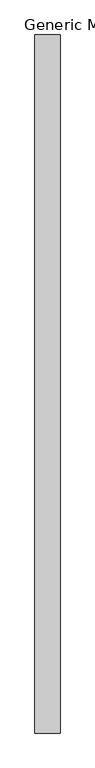
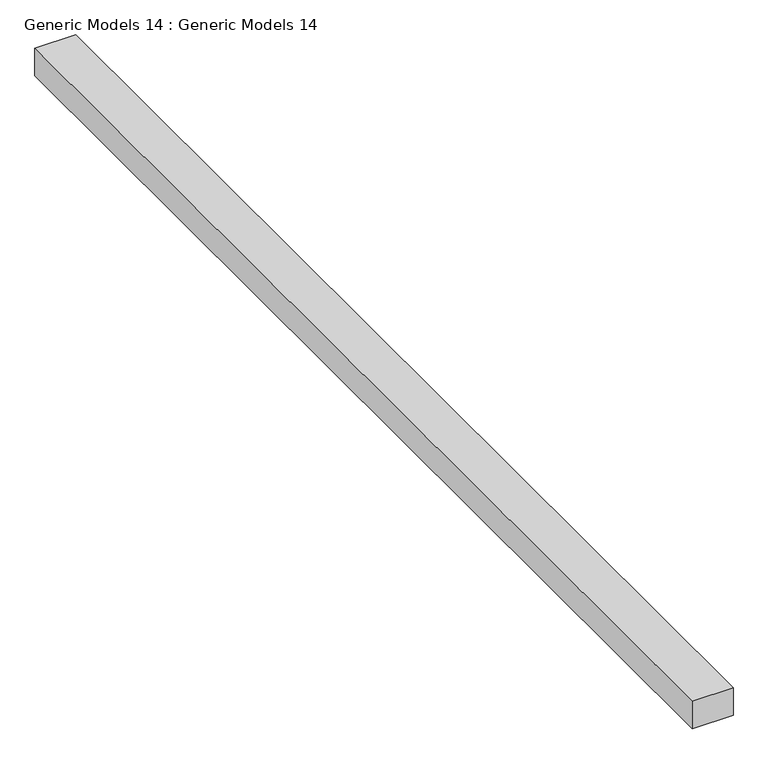
"""IFC4 building model written with IfcOpenShell, lengths in millimetres: proxy geometry, Generic Models 14 : Generic Models 14."""

from ifc_helpers import new_model, si_unit, frame, origin, place, context, project, spatial, polyline, outline, extrude, source, transform, mapped, element, save


def generic_models_14_generic_models_14_5b98b352(model_context):
    return source(origin(), model_context, "Body", "SweptSolid", [
        extrude(outline(polyline([(-12915.9319556, -4383.6963334), (-13347.7319556, -4383.6963334), (-13347.7319556, 7605.1036666), (-12915.9319556, 7605.1036666), (-12915.9319556, -4383.6963334)])), frame((0.0, 0.0, 29298.9561104), z_axis=(0.0, 0.0, 1.0), x_axis=(1.0, 0.0, 0.0)), (0.0, 0.0, 1.0), 304.8),
    ])


if __name__ == "__main__":
    model = new_model("IFC4")
    model_context = context("Model", 3, world=origin())
    ifc_project = project(units=[si_unit("LENGTHUNIT", "METRE", prefix="MILLI")], contexts=[model_context])
    site = spatial("IfcSite", under=ifc_project)
    building = spatial("IfcBuilding", under=site)
    placement = place(None, origin())
    generic_models_14_generic_models_14_shape = generic_models_14_generic_models_14_5b98b352(model_context)
    element("IfcBuildingElementProxy", 1, Name="Generic Models 14 : Generic Models 14", ObjectType="Generic Models 14 : Generic Models 14", at=placement, inside=building, context=model_context, shape_type="MappedRepresentation", body=[
        mapped(generic_models_14_generic_models_14_shape, transform((0.0, 0.0, 0.0), x_axis=(1.0, 0.0, 0.0), y_axis=(0.0, 1.0, 0.0), z_axis=(0.0, 0.0, 1.0))),
    ])
    save(model, "model.ifc")
